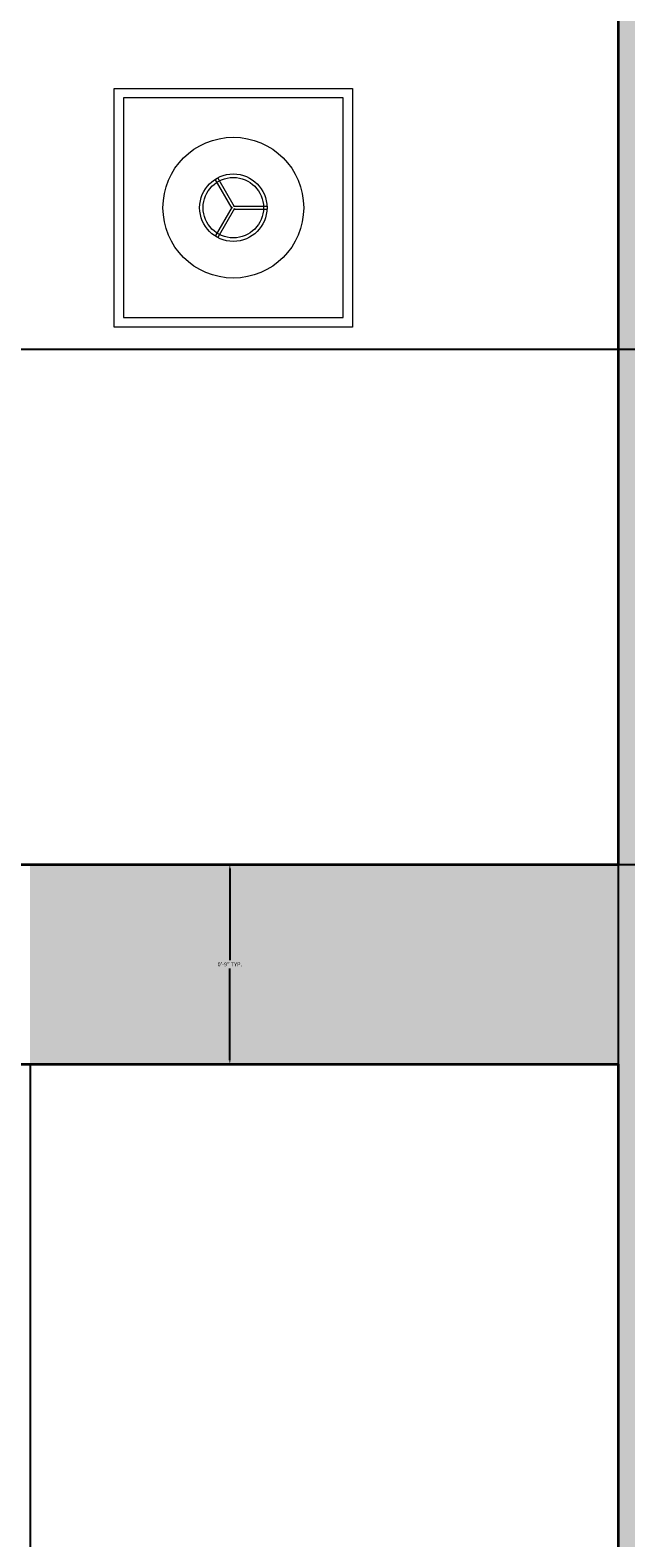
# Model space of a CAD drawing. Units: inches. Extents: x -5 to 330, y -522 to 40.
# Tile 17 of 23: x 246 to 272, y -447 to -380. Entities that reach past the tile are written whole.
import ezdxf

# ---------------------------------------------------------------- set-up
doc = ezdxf.new("R2010")
doc.units = ezdxf.units.IN
doc.header["$MEASUREMENT"] = 0
for name, color, linetype, lineweight in [('A-ANNO-DIMS', 2, 'Continuous', 18), ('A-FURN', 8, 'Continuous', 18), ('A-SITE-WALL', 7, 'Continuous', 35), ('A-WALL', 7, 'Continuous', 35)]:
    doc.layers.add(name, color=color, linetype=linetype, lineweight=lineweight)
doc.layers.add('A-WALL-PATT', color=18, linetype='Continuous', lineweight=13, true_color=0x000000)
doc.styles.get("Standard").update_dxf_attribs({"font": 'arial.ttf'})
doc.dimstyles.get("Standard").update_dxf_attribs({"dimtxt": 0.18, "dimasz": 0.18, "dimexe": 0.18, "dimexo": 0.0625, "dimgap": 0.09, "dimtad": 0, "dimtih": 1, "dimtoh": 1, "dimdec": 0, "dimzin": 0, "dimdsep": 46, "dimlunit": 3, "dimtxsty": 'Standard', "dimcen": 0.09, "dimadec": 0, "dimazin": 0, "dimtfac": 1, "dimtdec": 0, "dimtofl": 0, "dimtmove": 0, "dimatfit": 3, "dimfxl": 1, "dimtolj": 1, "dimtzin": 0, "dimarcsym": 0})

# ---------------------------------------------------------------- blocks, each defined once
blk = doc.blocks.new('END-TABLE-SQUARE')
for p, q in [((5.318, 5.343), (4.56, 6.656)), ((5.435, 5.41), (4.677, 6.724)), ((5.377, 5.444), (6.893, 5.444)), ((5.318, 5.41), (4.56, 4.097)), ((5.435, 5.343), (4.677, 4.029)), ((5.377, 5.309), (6.893, 5.309))]:
    blk.add_line(p, q)
at = {"ltscale": 0.03}
blk.add_lwpolyline([(0, 0), (0, 10.753), (10.753, 10.753), (10.753, 0)], close=True, dxfattribs=at)
blk.add_lwpolyline([(0.43, 10.323), (0.43, 0.43), (10.323, 0.43), (10.323, 10.323)], close=True)
for radius in [3.171, 1.518, 1.361]:
    blk.add_circle((5.377, 5.377), radius)
blk = doc.blocks.new('*D20')
at = {"layer": 'A-ANNO-DIMS', "color": 0, "lineweight": -2, "transparency": 16777216}
for p, q in [((245.572, -417.144), (254.69, -417.144)), ((254.51, -417.324), (254.51, -421.462)), ((254.51, -425.964), (254.51, -421.825)), ((245.572, -426.144), (254.69, -426.144))]:
    blk.add_line(p, q, dxfattribs=at)
at = {"layer": 'A-ANNO-DIMS', "color": 0, "transparency": 16777216}
for points in [[(254.48, -417.324), (254.54, -417.324), (254.51, -417.144)], [(254.48, -425.964), (254.54, -425.964), (254.51, -426.144)]]:
    blk.add_solid(points, dxfattribs=at)
at = {"layer": 'Defpoints', "color": 0, "transparency": 16777216}
for p in [(245.51, -417.144), (254.51, -417.144), (245.51, -426.144)]:
    blk.add_point(p, dxfattribs=at)
at = {"layer": 'A-ANNO-DIMS', "color": 0, "transparency": 16777216, "insert": (254.51, -421.644), "char_height": 0.18, "attachment_point": 5}
blk.add_mtext('\\A1;0\'-9" TYP.', dxfattribs=at)
blk = doc.blocks.new('*D37')
at = {"layer": 'A-ANNO-DIMS', "color": 0, "lineweight": -2, "transparency": 16777216}
for p, q in [((164.01, -53.206), (164.01, -522.309)), ((272.01, -53.206), (272.01, -522.309)), ((164.19, -522.129), (217.681, -522.129)), ((271.83, -522.129), (218.339, -522.129))]:
    blk.add_line(p, q, dxfattribs=at)
at = {"layer": 'A-ANNO-DIMS', "color": 0, "transparency": 16777216}
for points in [[(164.19, -522.099), (164.19, -522.159), (164.01, -522.129)], [(271.83, -522.099), (271.83, -522.159), (272.01, -522.129)]]:
    blk.add_solid(points, dxfattribs=at)
at = {"layer": 'Defpoints', "color": 0, "transparency": 16777216}
for p in [(164.01, -53.144), (272.01, -53.144), (272.01, -522.129)]:
    blk.add_point(p, dxfattribs=at)
at = {"layer": 'A-ANNO-DIMS', "color": 0, "transparency": 16777216, "insert": (218.01, -522.129), "char_height": 0.18, "attachment_point": 5}
blk.add_mtext('\\A1;9\'-0"', dxfattribs=at)
blk = doc.blocks.new('*D44')
at = {"layer": 'A-ANNO-DIMS', "color": 0, "lineweight": -2, "transparency": 16777216}
for p, q in [((128.572, -393.928), (308.175, -393.928)), ((307.995, -394.108), (307.995, -405.356)), ((307.995, -416.964), (307.995, -405.716)), ((128.572, -417.144), (308.175, -417.144))]:
    blk.add_line(p, q, dxfattribs=at)
at = {"layer": 'A-ANNO-DIMS', "color": 0, "transparency": 16777216}
for points in [[(307.965, -394.108), (308.025, -394.108), (307.995, -393.928)], [(307.965, -416.964), (308.025, -416.964), (307.995, -417.144)]]:
    blk.add_solid(points, dxfattribs=at)
at = {"layer": 'Defpoints', "color": 0, "transparency": 16777216}
for p in [(128.51, -393.928), (307.995, -393.928), (128.51, -417.144)]:
    blk.add_point(p, dxfattribs=at)
at = {"layer": 'A-ANNO-DIMS', "color": 0, "transparency": 16777216, "insert": (307.995, -405.536), "char_height": 0.18, "attachment_point": 5}
blk.add_mtext('\\A1;1\'-11"', dxfattribs=at)
blk = doc.blocks.new('*D46')
at = {"layer": 'A-ANNO-DIMS', "color": 0, "lineweight": -2, "transparency": 16777216}
for p, q in [((245.51, -426.206), (245.51, -522.309)), ((272.01, -426.206), (272.01, -522.309)), ((245.69, -522.129), (258.219, -522.129)), ((271.83, -522.129), (259.3, -522.129))]:
    blk.add_line(p, q, dxfattribs=at)
at = {"layer": 'A-ANNO-DIMS', "color": 0, "transparency": 16777216}
for points in [[(245.69, -522.099), (245.69, -522.159), (245.51, -522.129)], [(271.83, -522.099), (271.83, -522.159), (272.01, -522.129)]]:
    blk.add_solid(points, dxfattribs=at)
at = {"layer": 'Defpoints', "color": 0, "transparency": 16777216}
for p in [(245.51, -426.144), (272.01, -426.144), (272.01, -522.129)]:
    blk.add_point(p, dxfattribs=at)
at = {"layer": 'A-ANNO-DIMS', "color": 0, "transparency": 16777216, "insert": (258.76, -522.129), "char_height": 0.18, "attachment_point": 5}
blk.add_mtext('\\A1;2\'-2 1/2"', dxfattribs=at)

msp = doc.modelspace()

# ---------------------------------------------------------------- hatches: boundary and pattern name
at = {"layer": 'A-WALL-PATT'}
h = msp.add_hatch(color=256, dxfattribs=at)
h.dxf.hatch_style = 1
h.paths.add_polyline_path([(164.01, -44.152), (159.51, -44.152), (159.51, -153.144), (164.01, -153.144)], flags=17)
h.paths.add_polyline_path([(224.01, -188.144), (272.01, -188.144), (272.01, -218.144), (260.01, -218.144), (260.01, -222.644), (272.01, -222.644), (272.01, -292.644), (159.01, -292.644), (159.01, -297.144), (272.01, -297.144), (272.01, -417.144), (245.51, -417.144), (245.51, -426.144), (272.01, -426.144), (272.01, -495.144), (281.01, -495.144), (281.01, 12.356), (23.51, 12.356), (23.51, -426.144), (62.918, -426.144), (62.918, -417.144), (32.51, -417.144), (32.51, -297.144), (48.129, -297.144), (48.129, -292.644), (32.51, -292.644), (32.51, -140.644), (133.51, -140.644), (133.51, -131.644), (32.51, -131.644), (32.51, 3.356), (159.51, 3.356), (164.01, 3.356), (220.01, 3.356), (224.51, 3.356), (272.01, 3.356), (272.01, -179.144), (159.51, -179.144), (159.51, -188.144), (219.51, -188.144), (219.51, -266.644), (224.01, -266.644), (224.01, -222.644), (236.01, -222.644), (236.01, -218.144), (224.01, -218.144)])
h.paths.add_polyline_path([(133.01, -292.644), (128.51, -292.644), (128.51, -297.144), (128.51, -417.144), (122.918, -417.144), (122.918, -426.144), (133.01, -426.144)], flags=17)
h.paths.add_polyline_path([(185.51, -417.144), (159.01, -417.144), (159.01, -426.144), (185.51, -426.144)], flags=17)
h.paths.add_polyline_path([(133.51, -140.644), (129.01, -140.644), (129.01, -246.644), (133.51, -246.644)], flags=17)
h.paths.add_polyline_path([(246.01, -48.644), (224.51, -48.644), (224.51, -27.627), (220.01, -27.627), (220.01, -48.644), (198.604, -48.644), (198.604, -53.144), (246.01, -53.144)], flags=17)

# ---------------------------------------------------------------- linework, layer by layer
at = {"layer": 'A-SITE-WALL'}
msp.add_line((272.01, -426.144), (272.01, -495.144), dxfattribs=at)
at = {"layer": 'A-WALL'}
for p, q in [((272.01, -297.144), (272.01, -417.144)), ((159.01, -417.144), (272.01, -417.144)), ((159.01, -426.144), (272.01, -426.144))]:
    msp.add_line(p, q, dxfattribs=at)

# ---------------------------------------------------------------- block references
at = {"layer": 'A-FURN'}
msp.add_blockref('END-TABLE-SQUARE', (249.291, -392.932), dxfattribs=at)

# ---------------------------------------------------------------- dimensions: what is measured, and where the dimension line sits
at = {"layer": 'A-ANNO-DIMS'}
for p1, p2, picture, middle in [((164.01, -53.144), (272.01, -53.144), '*D37', (218.01, -522.129)), ((245.51, -426.144), (272.01, -426.144), '*D46', (258.76, -522.129))]:
    dim = msp.add_linear_dim(base=(272.01, -522.129), p1=p1, p2=p2, dimstyle='Standard', override={"dimdec": 1, "dimlfac": 1, "dimrnd": 0, "dimzin": 1, "dimdsep": 46, "dimlunit": 4, "dimfrac": 2}, dxfattribs=at)
    dim.commit()
    dim.dimension.update_dxf_attribs({"geometry": picture, "text_midpoint": middle})
dim = msp.add_linear_dim(base=(307.995, -393.928), p1=(128.51, -417.144), p2=(128.51, -393.928), angle=90, dimstyle='Standard', override={"dimdec": 1, "dimlfac": 1, "dimrnd": 0, "dimzin": 1, "dimdsep": 46, "dimlunit": 4, "dimfrac": 2}, dxfattribs=at)
dim.commit()
dim.dimension.update_dxf_attribs({"geometry": '*D44', "text_midpoint": (307.995, -405.536)})
dim = msp.add_linear_dim(base=(254.51, -417.144), p1=(245.51, -426.144), p2=(245.51, -417.144), angle=90, text='<> TYP.', dimstyle='Standard', override={"dimdec": 1, "dimlfac": 1, "dimrnd": 0, "dimzin": 1, "dimdsep": 46, "dimlunit": 4, "dimfrac": 2}, dxfattribs=at)
dim.commit()
dim.dimension.update_dxf_attribs({"geometry": '*D20', "text_midpoint": (254.51, -421.644)})

doc.saveas('drawing.dxf')
